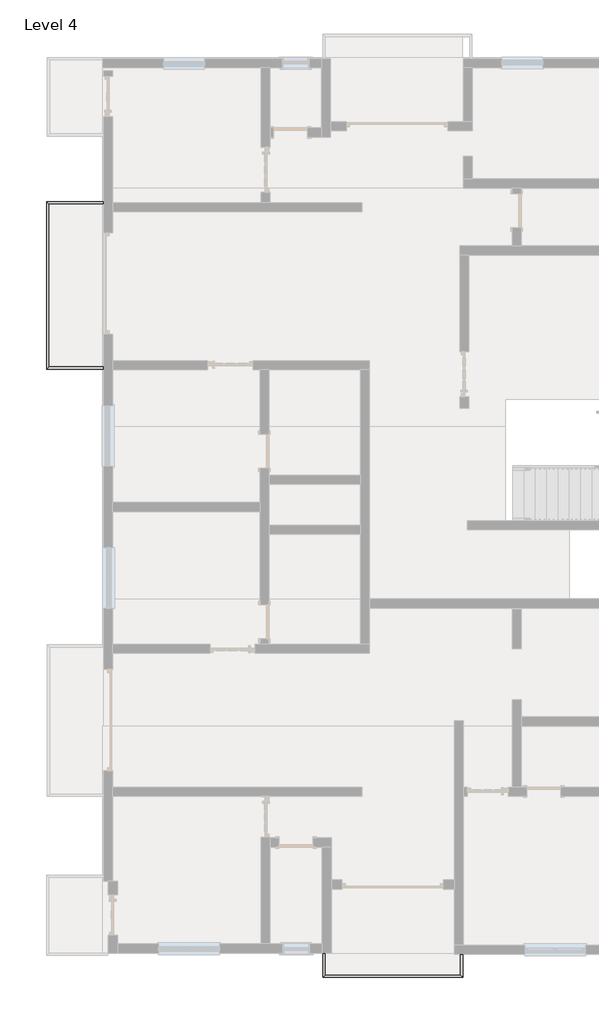
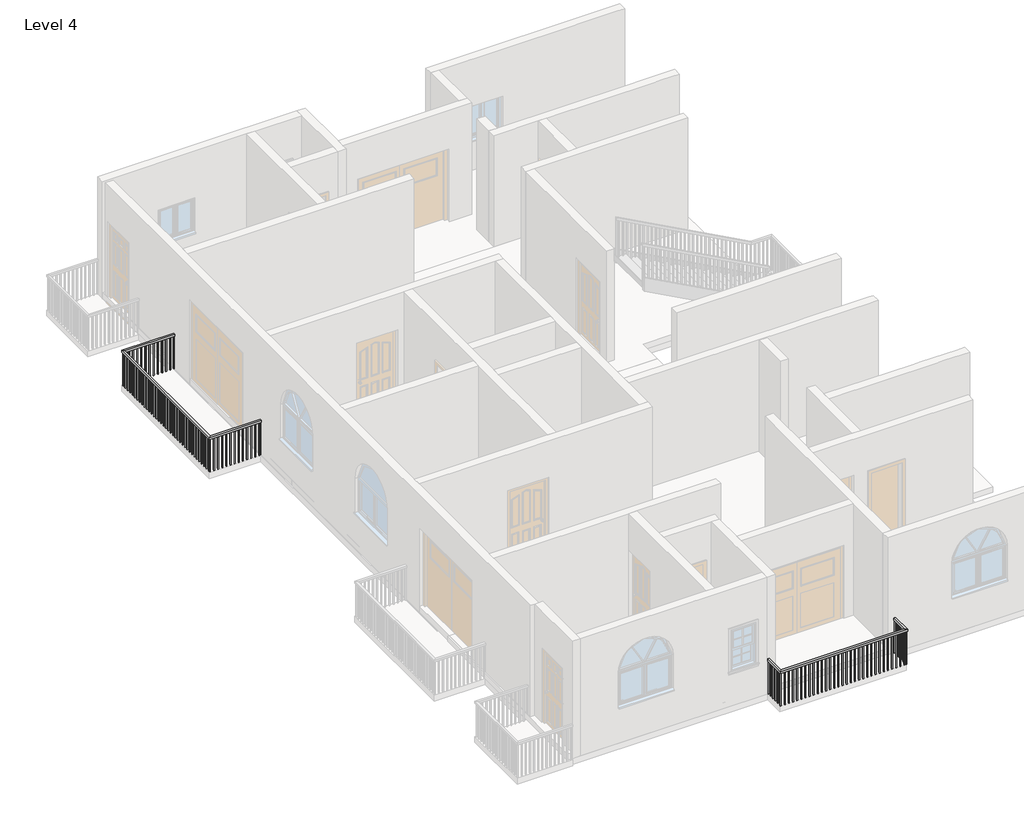
# One storey, part 4 of 7: 2 railings.
"""IFC4 building model written with IfcOpenShell, lengths in millimetres."""

from ifc_helpers import new_model, si_unit, frame, origin, place, context, project, spatial, polyline, outline, extrude, faceted_brep, element, save

model = new_model("IFC4")

# Units and contexts
model_context = context("Model", 3, world=origin())
ifc_project = project(units=[si_unit("LENGTHUNIT", "METRE", prefix="MILLI")], contexts=[model_context])

# Site, building, storey
site = spatial("IfcSite", under=ifc_project)
building = spatial("IfcBuilding", under=site)
storey = spatial("IfcBuildingStorey", under=building, Name="Level 4", Elevation=9144.0)

# Railings
placement = place(None, origin())
element("IfcRailing", 1, ObjectType="Handrail - Rectangular", at=placement, inside=storey, context=model_context, shape_type="SolidModel", body=[
    faceted_brep([(-1375.8109037, -10612.9037749, 10058.4), (-1375.8109037, -10612.9037749, 10007.6), (-1426.6109037, -10612.9037749, 10007.6), (-1426.6109037, -10612.9037749, 10058.4), (-1375.8109037, -11108.2037749, 10058.4), (-1375.8109037, -11108.2037749, 10007.6), (-1426.6109037, -11159.0037749, 10007.6), (-1426.6109037, -11159.0037749, 10058.4), (1659.4890963, -11108.2037749, 10058.4), (1659.4890963, -11108.2037749, 10007.6), (1710.2890963, -11159.0037749, 10007.6), (1710.2890963, -11159.0037749, 10058.4), (1659.4890963, -10638.3037749, 10058.4), (1710.2890963, -10638.3037749, 10058.4), (1710.2890963, -10638.3037749, 10007.6), (1659.4890963, -10638.3037749, 10007.6)], [[[0, 1, 2, 3]], [[1, 0, 4, 5]], [[2, 1, 5, 6]], [[3, 2, 6, 7]], [[0, 3, 7, 4]], [[5, 4, 8, 9]], [[6, 5, 9, 10]], [[7, 6, 10, 11]], [[4, 7, 11, 8]], [[12, 13, 14, 15]], [[9, 8, 12, 15]], [[10, 9, 15, 14]], [[11, 10, 14, 13]], [[8, 11, 13, 12]]]),
    extrude(outline(polyline([(1694.4140963, -10736.7287749), (1675.3640963, -10736.7287749), (1675.3640963, -10717.6787749), (1694.4140963, -10717.6787749), (1694.4140963, -10736.7287749)])), frame((0.0, 0.0, 9144.0), z_axis=(0.0, 0.0, 1.0), x_axis=(1.0, 0.0, 0.0)), (0.0, 0.0, 1.0), 863.6),
    extrude(outline(polyline([(1694.4140963, -10838.3287749), (1675.3640963, -10838.3287749), (1675.3640963, -10819.2787749), (1694.4140963, -10819.2787749), (1694.4140963, -10838.3287749)])), frame((0.0, 0.0, 9144.0), z_axis=(0.0, 0.0, 1.0), x_axis=(1.0, 0.0, 0.0)), (0.0, 0.0, 1.0), 863.6),
    extrude(outline(polyline([(1694.4140963, -10939.9287749), (1675.3640963, -10939.9287749), (1675.3640963, -10920.8787749), (1694.4140963, -10920.8787749), (1694.4140963, -10939.9287749)])), frame((0.0, 0.0, 9144.0), z_axis=(0.0, 0.0, 1.0), x_axis=(1.0, 0.0, 0.0)), (0.0, 0.0, 1.0), 863.6),
    extrude(outline(polyline([(1694.4140963, -11041.5287749), (1675.3640963, -11041.5287749), (1675.3640963, -11022.4787749), (1694.4140963, -11022.4787749), (1694.4140963, -11041.5287749)])), frame((0.0, 0.0, 9144.0), z_axis=(0.0, 0.0, 1.0), x_axis=(1.0, 0.0, 0.0)), (0.0, 0.0, 1.0), 863.6),
    extrude(outline(polyline([(1637.2640963, -11143.1287749), (1637.2640963, -11124.0787749), (1656.3140963, -11124.0787749), (1656.3140963, -11143.1287749), (1637.2640963, -11143.1287749)])), frame((0.0, 0.0, 9144.0), z_axis=(0.0, 0.0, 1.0), x_axis=(1.0, 0.0, 0.0)), (0.0, 0.0, 1.0), 863.6),
    extrude(outline(polyline([(1535.6640963, -11143.1287749), (1535.6640963, -11124.0787749), (1554.7140963, -11124.0787749), (1554.7140963, -11143.1287749), (1535.6640963, -11143.1287749)])), frame((0.0, 0.0, 9144.0), z_axis=(0.0, 0.0, 1.0), x_axis=(1.0, 0.0, 0.0)), (0.0, 0.0, 1.0), 863.6),
    extrude(outline(polyline([(1434.0640963, -11143.1287749), (1434.0640963, -11124.0787749), (1453.1140963, -11124.0787749), (1453.1140963, -11143.1287749), (1434.0640963, -11143.1287749)])), frame((0.0, 0.0, 9144.0), z_axis=(0.0, 0.0, 1.0), x_axis=(1.0, 0.0, 0.0)), (0.0, 0.0, 1.0), 863.6),
    extrude(outline(polyline([(1332.4640963, -11143.1287749), (1332.4640963, -11124.0787749), (1351.5140963, -11124.0787749), (1351.5140963, -11143.1287749), (1332.4640963, -11143.1287749)])), frame((0.0, 0.0, 9144.0), z_axis=(0.0, 0.0, 1.0), x_axis=(1.0, 0.0, 0.0)), (0.0, 0.0, 1.0), 863.6),
    extrude(outline(polyline([(1230.8640963, -11143.1287749), (1230.8640963, -11124.0787749), (1249.9140963, -11124.0787749), (1249.9140963, -11143.1287749), (1230.8640963, -11143.1287749)])), frame((0.0, 0.0, 9144.0), z_axis=(0.0, 0.0, 1.0), x_axis=(1.0, 0.0, 0.0)), (0.0, 0.0, 1.0), 863.6),
    extrude(outline(polyline([(1129.2640963, -11143.1287749), (1129.2640963, -11124.0787749), (1148.3140963, -11124.0787749), (1148.3140963, -11143.1287749), (1129.2640963, -11143.1287749)])), frame((0.0, 0.0, 9144.0), z_axis=(0.0, 0.0, 1.0), x_axis=(1.0, 0.0, 0.0)), (0.0, 0.0, 1.0), 863.6),
    extrude(outline(polyline([(1027.6640963, -11143.1287749), (1027.6640963, -11124.0787749), (1046.7140963, -11124.0787749), (1046.7140963, -11143.1287749), (1027.6640963, -11143.1287749)])), frame((0.0, 0.0, 9144.0), z_axis=(0.0, 0.0, 1.0), x_axis=(1.0, 0.0, 0.0)), (0.0, 0.0, 1.0), 863.6),
    extrude(outline(polyline([(926.0640963, -11143.1287749), (926.0640963, -11124.0787749), (945.1140963, -11124.0787749), (945.1140963, -11143.1287749), (926.0640963, -11143.1287749)])), frame((0.0, 0.0, 9144.0), z_axis=(0.0, 0.0, 1.0), x_axis=(1.0, 0.0, 0.0)), (0.0, 0.0, 1.0), 863.6),
    extrude(outline(polyline([(824.4640963, -11143.1287749), (824.4640963, -11124.0787749), (843.5140963, -11124.0787749), (843.5140963, -11143.1287749), (824.4640963, -11143.1287749)])), frame((0.0, 0.0, 9144.0), z_axis=(0.0, 0.0, 1.0), x_axis=(1.0, 0.0, 0.0)), (0.0, 0.0, 1.0), 863.6),
    extrude(outline(polyline([(722.8640963, -11143.1287749), (722.8640963, -11124.0787749), (741.9140963, -11124.0787749), (741.9140963, -11143.1287749), (722.8640963, -11143.1287749)])), frame((0.0, 0.0, 9144.0), z_axis=(0.0, 0.0, 1.0), x_axis=(1.0, 0.0, 0.0)), (0.0, 0.0, 1.0), 863.6),
    extrude(outline(polyline([(621.2640963, -11143.1287749), (621.2640963, -11124.0787749), (640.3140963, -11124.0787749), (640.3140963, -11143.1287749), (621.2640963, -11143.1287749)])), frame((0.0, 0.0, 9144.0), z_axis=(0.0, 0.0, 1.0), x_axis=(1.0, 0.0, 0.0)), (0.0, 0.0, 1.0), 863.6),
    extrude(outline(polyline([(519.6640963, -11143.1287749), (519.6640963, -11124.0787749), (538.7140963, -11124.0787749), (538.7140963, -11143.1287749), (519.6640963, -11143.1287749)])), frame((0.0, 0.0, 9144.0), z_axis=(0.0, 0.0, 1.0), x_axis=(1.0, 0.0, 0.0)), (0.0, 0.0, 1.0), 863.6),
    extrude(outline(polyline([(418.0640963, -11143.1287749), (418.0640963, -11124.0787749), (437.1140963, -11124.0787749), (437.1140963, -11143.1287749), (418.0640963, -11143.1287749)])), frame((0.0, 0.0, 9144.0), z_axis=(0.0, 0.0, 1.0), x_axis=(1.0, 0.0, 0.0)), (0.0, 0.0, 1.0), 863.6),
    extrude(outline(polyline([(316.4640963, -11143.1287749), (316.4640963, -11124.0787749), (335.5140963, -11124.0787749), (335.5140963, -11143.1287749), (316.4640963, -11143.1287749)])), frame((0.0, 0.0, 9144.0), z_axis=(0.0, 0.0, 1.0), x_axis=(1.0, 0.0, 0.0)), (0.0, 0.0, 1.0), 863.6),
    extrude(outline(polyline([(214.8640963, -11143.1287749), (214.8640963, -11124.0787749), (233.9140963, -11124.0787749), (233.9140963, -11143.1287749), (214.8640963, -11143.1287749)])), frame((0.0, 0.0, 9144.0), z_axis=(0.0, 0.0, 1.0), x_axis=(1.0, 0.0, 0.0)), (0.0, 0.0, 1.0), 863.6),
    extrude(outline(polyline([(113.2640963, -11143.1287749), (113.2640963, -11124.0787749), (132.3140963, -11124.0787749), (132.3140963, -11143.1287749), (113.2640963, -11143.1287749)])), frame((0.0, 0.0, 9144.0), z_axis=(0.0, 0.0, 1.0), x_axis=(1.0, 0.0, 0.0)), (0.0, 0.0, 1.0), 863.6),
    extrude(outline(polyline([(11.6640963, -11143.1287749), (11.6640963, -11124.0787749), (30.7140963, -11124.0787749), (30.7140963, -11143.1287749), (11.6640963, -11143.1287749)])), frame((0.0, 0.0, 9144.0), z_axis=(0.0, 0.0, 1.0), x_axis=(1.0, 0.0, 0.0)), (0.0, 0.0, 1.0), 863.6),
    extrude(outline(polyline([(-89.9359037, -11143.1287749), (-89.9359037, -11124.0787749), (-70.8859037, -11124.0787749), (-70.8859037, -11143.1287749), (-89.9359037, -11143.1287749)])), frame((0.0, 0.0, 9144.0), z_axis=(0.0, 0.0, 1.0), x_axis=(1.0, 0.0, 0.0)), (0.0, 0.0, 1.0), 863.6),
    extrude(outline(polyline([(-191.5359037, -11143.1287749), (-191.5359037, -11124.0787749), (-172.4859037, -11124.0787749), (-172.4859037, -11143.1287749), (-191.5359037, -11143.1287749)])), frame((0.0, 0.0, 9144.0), z_axis=(0.0, 0.0, 1.0), x_axis=(1.0, 0.0, 0.0)), (0.0, 0.0, 1.0), 863.6),
    extrude(outline(polyline([(-293.1359037, -11143.1287749), (-293.1359037, -11124.0787749), (-274.0859037, -11124.0787749), (-274.0859037, -11143.1287749), (-293.1359037, -11143.1287749)])), frame((0.0, 0.0, 9144.0), z_axis=(0.0, 0.0, 1.0), x_axis=(1.0, 0.0, 0.0)), (0.0, 0.0, 1.0), 863.6),
    extrude(outline(polyline([(-394.7359037, -11143.1287749), (-394.7359037, -11124.0787749), (-375.6859037, -11124.0787749), (-375.6859037, -11143.1287749), (-394.7359037, -11143.1287749)])), frame((0.0, 0.0, 9144.0), z_axis=(0.0, 0.0, 1.0), x_axis=(1.0, 0.0, 0.0)), (0.0, 0.0, 1.0), 863.6),
    extrude(outline(polyline([(-496.3359037, -11143.1287749), (-496.3359037, -11124.0787749), (-477.2859037, -11124.0787749), (-477.2859037, -11143.1287749), (-496.3359037, -11143.1287749)])), frame((0.0, 0.0, 9144.0), z_axis=(0.0, 0.0, 1.0), x_axis=(1.0, 0.0, 0.0)), (0.0, 0.0, 1.0), 863.6),
    extrude(outline(polyline([(-597.9359037, -11143.1287749), (-597.9359037, -11124.0787749), (-578.8859037, -11124.0787749), (-578.8859037, -11143.1287749), (-597.9359037, -11143.1287749)])), frame((0.0, 0.0, 9144.0), z_axis=(0.0, 0.0, 1.0), x_axis=(1.0, 0.0, 0.0)), (0.0, 0.0, 1.0), 863.6),
    extrude(outline(polyline([(-699.5359037, -11143.1287749), (-699.5359037, -11124.0787749), (-680.4859037, -11124.0787749), (-680.4859037, -11143.1287749), (-699.5359037, -11143.1287749)])), frame((0.0, 0.0, 9144.0), z_axis=(0.0, 0.0, 1.0), x_axis=(1.0, 0.0, 0.0)), (0.0, 0.0, 1.0), 863.6),
    extrude(outline(polyline([(-801.1359037, -11143.1287749), (-801.1359037, -11124.0787749), (-782.0859037, -11124.0787749), (-782.0859037, -11143.1287749), (-801.1359037, -11143.1287749)])), frame((0.0, 0.0, 9144.0), z_axis=(0.0, 0.0, 1.0), x_axis=(1.0, 0.0, 0.0)), (0.0, 0.0, 1.0), 863.6),
    extrude(outline(polyline([(-902.7359037, -11143.1287749), (-902.7359037, -11124.0787749), (-883.6859037, -11124.0787749), (-883.6859037, -11143.1287749), (-902.7359037, -11143.1287749)])), frame((0.0, 0.0, 9144.0), z_axis=(0.0, 0.0, 1.0), x_axis=(1.0, 0.0, 0.0)), (0.0, 0.0, 1.0), 863.6),
    extrude(outline(polyline([(-1004.3359037, -11143.1287749), (-1004.3359037, -11124.0787749), (-985.2859037, -11124.0787749), (-985.2859037, -11143.1287749), (-1004.3359037, -11143.1287749)])), frame((0.0, 0.0, 9144.0), z_axis=(0.0, 0.0, 1.0), x_axis=(1.0, 0.0, 0.0)), (0.0, 0.0, 1.0), 863.6),
    extrude(outline(polyline([(-1105.9359037, -11143.1287749), (-1105.9359037, -11124.0787749), (-1086.8859037, -11124.0787749), (-1086.8859037, -11143.1287749), (-1105.9359037, -11143.1287749)])), frame((0.0, 0.0, 9144.0), z_axis=(0.0, 0.0, 1.0), x_axis=(1.0, 0.0, 0.0)), (0.0, 0.0, 1.0), 863.6),
    extrude(outline(polyline([(-1207.5359037, -11143.1287749), (-1207.5359037, -11124.0787749), (-1188.4859037, -11124.0787749), (-1188.4859037, -11143.1287749), (-1207.5359037, -11143.1287749)])), frame((0.0, 0.0, 9144.0), z_axis=(0.0, 0.0, 1.0), x_axis=(1.0, 0.0, 0.0)), (0.0, 0.0, 1.0), 863.6),
    extrude(outline(polyline([(-1309.1359037, -11143.1287749), (-1309.1359037, -11124.0787749), (-1290.0859037, -11124.0787749), (-1290.0859037, -11143.1287749), (-1309.1359037, -11143.1287749)])), frame((0.0, 0.0, 9144.0), z_axis=(0.0, 0.0, 1.0), x_axis=(1.0, 0.0, 0.0)), (0.0, 0.0, 1.0), 863.6),
    extrude(outline(polyline([(-1410.7359037, -11111.3787749), (-1391.6859037, -11111.3787749), (-1391.6859037, -11130.4287749), (-1410.7359037, -11130.4287749), (-1410.7359037, -11111.3787749)])), frame((0.0, 0.0, 9144.0), z_axis=(0.0, 0.0, 1.0), x_axis=(1.0, 0.0, 0.0)), (0.0, 0.0, 1.0), 863.6),
    extrude(outline(polyline([(-1410.7359037, -11009.7787749), (-1391.6859037, -11009.7787749), (-1391.6859037, -11028.8287749), (-1410.7359037, -11028.8287749), (-1410.7359037, -11009.7787749)])), frame((0.0, 0.0, 9144.0), z_axis=(0.0, 0.0, 1.0), x_axis=(1.0, 0.0, 0.0)), (0.0, 0.0, 1.0), 863.6),
    extrude(outline(polyline([(-1410.7359037, -10908.1787749), (-1391.6859037, -10908.1787749), (-1391.6859037, -10927.2287749), (-1410.7359037, -10927.2287749), (-1410.7359037, -10908.1787749)])), frame((0.0, 0.0, 9144.0), z_axis=(0.0, 0.0, 1.0), x_axis=(1.0, 0.0, 0.0)), (0.0, 0.0, 1.0), 863.6),
    extrude(outline(polyline([(-1410.7359037, -10806.5787749), (-1391.6859037, -10806.5787749), (-1391.6859037, -10825.6287749), (-1410.7359037, -10825.6287749), (-1410.7359037, -10806.5787749)])), frame((0.0, 0.0, 9144.0), z_axis=(0.0, 0.0, 1.0), x_axis=(1.0, 0.0, 0.0)), (0.0, 0.0, 1.0), 863.6),
    extrude(outline(polyline([(-1410.7359037, -10704.9787749), (-1391.6859037, -10704.9787749), (-1391.6859037, -10724.0287749), (-1410.7359037, -10724.0287749), (-1410.7359037, -10704.9787749)])), frame((0.0, 0.0, 9144.0), z_axis=(0.0, 0.0, 1.0), x_axis=(1.0, 0.0, 0.0)), (0.0, 0.0, 1.0), 863.6),
    extrude(outline(polyline([(1675.3640963, -11143.1287749), (1675.3640963, -11124.0787749), (1694.4140963, -11124.0787749), (1694.4140963, -11143.1287749), (1675.3640963, -11143.1287749)])), frame((0.0, 0.0, 9144.0), z_axis=(0.0, 0.0, 1.0), x_axis=(1.0, 0.0, 0.0)), (0.0, 0.0, 1.0), 863.6),
    extrude(outline(polyline([(-1410.7359037, -11124.0787749), (-1391.6859037, -11124.0787749), (-1391.6859037, -11143.1287749), (-1410.7359037, -11143.1287749), (-1410.7359037, -11124.0787749)])), frame((0.0, 0.0, 9144.0), z_axis=(0.0, 0.0, 1.0), x_axis=(1.0, 0.0, 0.0)), (0.0, 0.0, 1.0), 863.6),
    extrude(outline(polyline([(1694.4140963, -10657.3537749), (1675.3640963, -10657.3537749), (1675.3640963, -10638.3037749), (1694.4140963, -10638.3037749), (1694.4140963, -10657.3537749)])), frame((0.0, 0.0, 9144.0), z_axis=(0.0, 0.0, 1.0), x_axis=(1.0, 0.0, 0.0)), (0.0, 0.0, 1.0), 863.6),
    extrude(outline(polyline([(-1410.7359037, -10612.9037749), (-1391.6859037, -10612.9037749), (-1391.6859037, -10631.9537749), (-1410.7359037, -10631.9537749), (-1410.7359037, -10612.9037749)])), frame((0.0, 0.0, 9144.0), z_axis=(0.0, 0.0, 1.0), x_axis=(1.0, 0.0, 0.0)), (0.0, 0.0, 1.0), 863.6),
])
element("IfcRailing", 2, ObjectType="Handrail - Rectangular", at=placement, inside=storey, context=model_context, shape_type="SolidModel", body=[
    faceted_brep([(-6330.8013636, 6151.0962251, 10058.4), (-6330.8013636, 6151.0962251, 10007.6), (-6330.8013636, 6201.8962251, 10007.6), (-6330.8013636, 6201.8962251, 10058.4), (-7563.8859037, 6151.0962251, 10058.4), (-7563.8859037, 6151.0962251, 10007.6), (-7614.6859037, 6201.8962251, 10007.6), (-7614.6859037, 6201.8962251, 10058.4), (-7563.8859037, 2506.1962251, 10058.4), (-7563.8859037, 2506.1962251, 10007.6), (-7614.6859037, 2455.3962251, 10007.6), (-7614.6859037, 2455.3962251, 10058.4), (-6330.8013636, 2506.1962251, 10058.4), (-6330.8013636, 2455.3962251, 10058.4), (-6330.8013636, 2455.3962251, 10007.6), (-6330.8013636, 2506.1962251, 10007.6)], [[[0, 1, 2, 3]], [[1, 0, 4, 5]], [[2, 1, 5, 6]], [[3, 2, 6, 7]], [[0, 3, 7, 4]], [[5, 4, 8, 9]], [[6, 5, 9, 10]], [[7, 6, 10, 11]], [[4, 7, 11, 8]], [[12, 13, 14, 15]], [[9, 8, 12, 15]], [[10, 9, 15, 14]], [[11, 10, 14, 13]], [[8, 11, 13, 12]]]),
    extrude(outline(polyline([(-6379.6109037, 2471.2712251), (-6379.6109037, 2490.3212251), (-6360.5609037, 2490.3212251), (-6360.5609037, 2471.2712251), (-6379.6109037, 2471.2712251)])), frame((0.0, 0.0, 9144.0), z_axis=(0.0, 0.0, 1.0), x_axis=(1.0, 0.0, 0.0)), (0.0, 0.0, 1.0), 863.6),
    extrude(outline(polyline([(-6481.2109037, 2471.2712251), (-6481.2109037, 2490.3212251), (-6462.1609037, 2490.3212251), (-6462.1609037, 2471.2712251), (-6481.2109037, 2471.2712251)])), frame((0.0, 0.0, 9144.0), z_axis=(0.0, 0.0, 1.0), x_axis=(1.0, 0.0, 0.0)), (0.0, 0.0, 1.0), 863.6),
    extrude(outline(polyline([(-6582.8109037, 2471.2712251), (-6582.8109037, 2490.3212251), (-6563.7609037, 2490.3212251), (-6563.7609037, 2471.2712251), (-6582.8109037, 2471.2712251)])), frame((0.0, 0.0, 9144.0), z_axis=(0.0, 0.0, 1.0), x_axis=(1.0, 0.0, 0.0)), (0.0, 0.0, 1.0), 863.6),
    extrude(outline(polyline([(-6684.4109037, 2471.2712251), (-6684.4109037, 2490.3212251), (-6665.3609037, 2490.3212251), (-6665.3609037, 2471.2712251), (-6684.4109037, 2471.2712251)])), frame((0.0, 0.0, 9144.0), z_axis=(0.0, 0.0, 1.0), x_axis=(1.0, 0.0, 0.0)), (0.0, 0.0, 1.0), 863.6),
    extrude(outline(polyline([(-6786.0109037, 2471.2712251), (-6786.0109037, 2490.3212251), (-6766.9609037, 2490.3212251), (-6766.9609037, 2471.2712251), (-6786.0109037, 2471.2712251)])), frame((0.0, 0.0, 9144.0), z_axis=(0.0, 0.0, 1.0), x_axis=(1.0, 0.0, 0.0)), (0.0, 0.0, 1.0), 863.6),
    extrude(outline(polyline([(-6887.6109037, 2471.2712251), (-6887.6109037, 2490.3212251), (-6868.5609037, 2490.3212251), (-6868.5609037, 2471.2712251), (-6887.6109037, 2471.2712251)])), frame((0.0, 0.0, 9144.0), z_axis=(0.0, 0.0, 1.0), x_axis=(1.0, 0.0, 0.0)), (0.0, 0.0, 1.0), 863.6),
    extrude(outline(polyline([(-6989.2109037, 2471.2712251), (-6989.2109037, 2490.3212251), (-6970.1609037, 2490.3212251), (-6970.1609037, 2471.2712251), (-6989.2109037, 2471.2712251)])), frame((0.0, 0.0, 9144.0), z_axis=(0.0, 0.0, 1.0), x_axis=(1.0, 0.0, 0.0)), (0.0, 0.0, 1.0), 863.6),
    extrude(outline(polyline([(-7090.8109037, 2471.2712251), (-7090.8109037, 2490.3212251), (-7071.7609037, 2490.3212251), (-7071.7609037, 2471.2712251), (-7090.8109037, 2471.2712251)])), frame((0.0, 0.0, 9144.0), z_axis=(0.0, 0.0, 1.0), x_axis=(1.0, 0.0, 0.0)), (0.0, 0.0, 1.0), 863.6),
    extrude(outline(polyline([(-7192.4109037, 2471.2712251), (-7192.4109037, 2490.3212251), (-7173.3609037, 2490.3212251), (-7173.3609037, 2471.2712251), (-7192.4109037, 2471.2712251)])), frame((0.0, 0.0, 9144.0), z_axis=(0.0, 0.0, 1.0), x_axis=(1.0, 0.0, 0.0)), (0.0, 0.0, 1.0), 863.6),
    extrude(outline(polyline([(-7294.0109037, 2471.2712251), (-7294.0109037, 2490.3212251), (-7274.9609037, 2490.3212251), (-7274.9609037, 2471.2712251), (-7294.0109037, 2471.2712251)])), frame((0.0, 0.0, 9144.0), z_axis=(0.0, 0.0, 1.0), x_axis=(1.0, 0.0, 0.0)), (0.0, 0.0, 1.0), 863.6),
    extrude(outline(polyline([(-7395.6109037, 2471.2712251), (-7395.6109037, 2490.3212251), (-7376.5609037, 2490.3212251), (-7376.5609037, 2471.2712251), (-7395.6109037, 2471.2712251)])), frame((0.0, 0.0, 9144.0), z_axis=(0.0, 0.0, 1.0), x_axis=(1.0, 0.0, 0.0)), (0.0, 0.0, 1.0), 863.6),
    extrude(outline(polyline([(-7497.2109037, 2471.2712251), (-7497.2109037, 2490.3212251), (-7478.1609037, 2490.3212251), (-7478.1609037, 2471.2712251), (-7497.2109037, 2471.2712251)])), frame((0.0, 0.0, 9144.0), z_axis=(0.0, 0.0, 1.0), x_axis=(1.0, 0.0, 0.0)), (0.0, 0.0, 1.0), 863.6),
    extrude(outline(polyline([(-7598.8109037, 2528.4212251), (-7579.7609037, 2528.4212251), (-7579.7609037, 2509.3712251), (-7598.8109037, 2509.3712251), (-7598.8109037, 2528.4212251)])), frame((0.0, 0.0, 9144.0), z_axis=(0.0, 0.0, 1.0), x_axis=(1.0, 0.0, 0.0)), (0.0, 0.0, 1.0), 863.6),
    extrude(outline(polyline([(-7598.8109037, 2630.0212251), (-7579.7609037, 2630.0212251), (-7579.7609037, 2610.9712251), (-7598.8109037, 2610.9712251), (-7598.8109037, 2630.0212251)])), frame((0.0, 0.0, 9144.0), z_axis=(0.0, 0.0, 1.0), x_axis=(1.0, 0.0, 0.0)), (0.0, 0.0, 1.0), 863.6),
    extrude(outline(polyline([(-7598.8109037, 2731.6212251), (-7579.7609037, 2731.6212251), (-7579.7609037, 2712.5712251), (-7598.8109037, 2712.5712251), (-7598.8109037, 2731.6212251)])), frame((0.0, 0.0, 9144.0), z_axis=(0.0, 0.0, 1.0), x_axis=(1.0, 0.0, 0.0)), (0.0, 0.0, 1.0), 863.6),
    extrude(outline(polyline([(-7598.8109037, 2833.2212251), (-7579.7609037, 2833.2212251), (-7579.7609037, 2814.1712251), (-7598.8109037, 2814.1712251), (-7598.8109037, 2833.2212251)])), frame((0.0, 0.0, 9144.0), z_axis=(0.0, 0.0, 1.0), x_axis=(1.0, 0.0, 0.0)), (0.0, 0.0, 1.0), 863.6),
    extrude(outline(polyline([(-7598.8109037, 2934.8212251), (-7579.7609037, 2934.8212251), (-7579.7609037, 2915.7712251), (-7598.8109037, 2915.7712251), (-7598.8109037, 2934.8212251)])), frame((0.0, 0.0, 9144.0), z_axis=(0.0, 0.0, 1.0), x_axis=(1.0, 0.0, 0.0)), (0.0, 0.0, 1.0), 863.6),
    extrude(outline(polyline([(-7598.8109037, 3036.4212251), (-7579.7609037, 3036.4212251), (-7579.7609037, 3017.3712251), (-7598.8109037, 3017.3712251), (-7598.8109037, 3036.4212251)])), frame((0.0, 0.0, 9144.0), z_axis=(0.0, 0.0, 1.0), x_axis=(1.0, 0.0, 0.0)), (0.0, 0.0, 1.0), 863.6),
    extrude(outline(polyline([(-7598.8109037, 3138.0212251), (-7579.7609037, 3138.0212251), (-7579.7609037, 3118.9712251), (-7598.8109037, 3118.9712251), (-7598.8109037, 3138.0212251)])), frame((0.0, 0.0, 9144.0), z_axis=(0.0, 0.0, 1.0), x_axis=(1.0, 0.0, 0.0)), (0.0, 0.0, 1.0), 863.6),
    extrude(outline(polyline([(-7598.8109037, 3239.6212251), (-7579.7609037, 3239.6212251), (-7579.7609037, 3220.5712251), (-7598.8109037, 3220.5712251), (-7598.8109037, 3239.6212251)])), frame((0.0, 0.0, 9144.0), z_axis=(0.0, 0.0, 1.0), x_axis=(1.0, 0.0, 0.0)), (0.0, 0.0, 1.0), 863.6),
    extrude(outline(polyline([(-7598.8109037, 3341.2212251), (-7579.7609037, 3341.2212251), (-7579.7609037, 3322.1712251), (-7598.8109037, 3322.1712251), (-7598.8109037, 3341.2212251)])), frame((0.0, 0.0, 9144.0), z_axis=(0.0, 0.0, 1.0), x_axis=(1.0, 0.0, 0.0)), (0.0, 0.0, 1.0), 863.6),
    extrude(outline(polyline([(-7598.8109037, 3442.8212251), (-7579.7609037, 3442.8212251), (-7579.7609037, 3423.7712251), (-7598.8109037, 3423.7712251), (-7598.8109037, 3442.8212251)])), frame((0.0, 0.0, 9144.0), z_axis=(0.0, 0.0, 1.0), x_axis=(1.0, 0.0, 0.0)), (0.0, 0.0, 1.0), 863.6),
    extrude(outline(polyline([(-7598.8109037, 3544.4212251), (-7579.7609037, 3544.4212251), (-7579.7609037, 3525.3712251), (-7598.8109037, 3525.3712251), (-7598.8109037, 3544.4212251)])), frame((0.0, 0.0, 9144.0), z_axis=(0.0, 0.0, 1.0), x_axis=(1.0, 0.0, 0.0)), (0.0, 0.0, 1.0), 863.6),
    extrude(outline(polyline([(-7598.8109037, 3646.0212251), (-7579.7609037, 3646.0212251), (-7579.7609037, 3626.9712251), (-7598.8109037, 3626.9712251), (-7598.8109037, 3646.0212251)])), frame((0.0, 0.0, 9144.0), z_axis=(0.0, 0.0, 1.0), x_axis=(1.0, 0.0, 0.0)), (0.0, 0.0, 1.0), 863.6),
    extrude(outline(polyline([(-7598.8109037, 3747.6212251), (-7579.7609037, 3747.6212251), (-7579.7609037, 3728.5712251), (-7598.8109037, 3728.5712251), (-7598.8109037, 3747.6212251)])), frame((0.0, 0.0, 9144.0), z_axis=(0.0, 0.0, 1.0), x_axis=(1.0, 0.0, 0.0)), (0.0, 0.0, 1.0), 863.6),
    extrude(outline(polyline([(-7598.8109037, 3849.2212251), (-7579.7609037, 3849.2212251), (-7579.7609037, 3830.1712251), (-7598.8109037, 3830.1712251), (-7598.8109037, 3849.2212251)])), frame((0.0, 0.0, 9144.0), z_axis=(0.0, 0.0, 1.0), x_axis=(1.0, 0.0, 0.0)), (0.0, 0.0, 1.0), 863.6),
    extrude(outline(polyline([(-7598.8109037, 3950.8212251), (-7579.7609037, 3950.8212251), (-7579.7609037, 3931.7712251), (-7598.8109037, 3931.7712251), (-7598.8109037, 3950.8212251)])), frame((0.0, 0.0, 9144.0), z_axis=(0.0, 0.0, 1.0), x_axis=(1.0, 0.0, 0.0)), (0.0, 0.0, 1.0), 863.6),
    extrude(outline(polyline([(-7598.8109037, 4052.4212251), (-7579.7609037, 4052.4212251), (-7579.7609037, 4033.3712251), (-7598.8109037, 4033.3712251), (-7598.8109037, 4052.4212251)])), frame((0.0, 0.0, 9144.0), z_axis=(0.0, 0.0, 1.0), x_axis=(1.0, 0.0, 0.0)), (0.0, 0.0, 1.0), 863.6),
    extrude(outline(polyline([(-7598.8109037, 4154.0212251), (-7579.7609037, 4154.0212251), (-7579.7609037, 4134.9712251), (-7598.8109037, 4134.9712251), (-7598.8109037, 4154.0212251)])), frame((0.0, 0.0, 9144.0), z_axis=(0.0, 0.0, 1.0), x_axis=(1.0, 0.0, 0.0)), (0.0, 0.0, 1.0), 863.6),
    extrude(outline(polyline([(-7598.8109037, 4255.6212251), (-7579.7609037, 4255.6212251), (-7579.7609037, 4236.5712251), (-7598.8109037, 4236.5712251), (-7598.8109037, 4255.6212251)])), frame((0.0, 0.0, 9144.0), z_axis=(0.0, 0.0, 1.0), x_axis=(1.0, 0.0, 0.0)), (0.0, 0.0, 1.0), 863.6),
    extrude(outline(polyline([(-7598.8109037, 4357.2212251), (-7579.7609037, 4357.2212251), (-7579.7609037, 4338.1712251), (-7598.8109037, 4338.1712251), (-7598.8109037, 4357.2212251)])), frame((0.0, 0.0, 9144.0), z_axis=(0.0, 0.0, 1.0), x_axis=(1.0, 0.0, 0.0)), (0.0, 0.0, 1.0), 863.6),
    extrude(outline(polyline([(-7598.8109037, 4458.8212251), (-7579.7609037, 4458.8212251), (-7579.7609037, 4439.7712251), (-7598.8109037, 4439.7712251), (-7598.8109037, 4458.8212251)])), frame((0.0, 0.0, 9144.0), z_axis=(0.0, 0.0, 1.0), x_axis=(1.0, 0.0, 0.0)), (0.0, 0.0, 1.0), 863.6),
    extrude(outline(polyline([(-7598.8109037, 4560.4212251), (-7579.7609037, 4560.4212251), (-7579.7609037, 4541.3712251), (-7598.8109037, 4541.3712251), (-7598.8109037, 4560.4212251)])), frame((0.0, 0.0, 9144.0), z_axis=(0.0, 0.0, 1.0), x_axis=(1.0, 0.0, 0.0)), (0.0, 0.0, 1.0), 863.6),
    extrude(outline(polyline([(-7598.8109037, 4662.0212251), (-7579.7609037, 4662.0212251), (-7579.7609037, 4642.9712251), (-7598.8109037, 4642.9712251), (-7598.8109037, 4662.0212251)])), frame((0.0, 0.0, 9144.0), z_axis=(0.0, 0.0, 1.0), x_axis=(1.0, 0.0, 0.0)), (0.0, 0.0, 1.0), 863.6),
    extrude(outline(polyline([(-7598.8109037, 4763.6212251), (-7579.7609037, 4763.6212251), (-7579.7609037, 4744.5712251), (-7598.8109037, 4744.5712251), (-7598.8109037, 4763.6212251)])), frame((0.0, 0.0, 9144.0), z_axis=(0.0, 0.0, 1.0), x_axis=(1.0, 0.0, 0.0)), (0.0, 0.0, 1.0), 863.6),
    extrude(outline(polyline([(-7598.8109037, 4865.2212251), (-7579.7609037, 4865.2212251), (-7579.7609037, 4846.1712251), (-7598.8109037, 4846.1712251), (-7598.8109037, 4865.2212251)])), frame((0.0, 0.0, 9144.0), z_axis=(0.0, 0.0, 1.0), x_axis=(1.0, 0.0, 0.0)), (0.0, 0.0, 1.0), 863.6),
    extrude(outline(polyline([(-7598.8109037, 4966.8212251), (-7579.7609037, 4966.8212251), (-7579.7609037, 4947.7712251), (-7598.8109037, 4947.7712251), (-7598.8109037, 4966.8212251)])), frame((0.0, 0.0, 9144.0), z_axis=(0.0, 0.0, 1.0), x_axis=(1.0, 0.0, 0.0)), (0.0, 0.0, 1.0), 863.6),
    extrude(outline(polyline([(-7598.8109037, 5068.4212251), (-7579.7609037, 5068.4212251), (-7579.7609037, 5049.3712251), (-7598.8109037, 5049.3712251), (-7598.8109037, 5068.4212251)])), frame((0.0, 0.0, 9144.0), z_axis=(0.0, 0.0, 1.0), x_axis=(1.0, 0.0, 0.0)), (0.0, 0.0, 1.0), 863.6),
    extrude(outline(polyline([(-7598.8109037, 5170.0212251), (-7579.7609037, 5170.0212251), (-7579.7609037, 5150.9712251), (-7598.8109037, 5150.9712251), (-7598.8109037, 5170.0212251)])), frame((0.0, 0.0, 9144.0), z_axis=(0.0, 0.0, 1.0), x_axis=(1.0, 0.0, 0.0)), (0.0, 0.0, 1.0), 863.6),
    extrude(outline(polyline([(-7598.8109037, 5271.6212251), (-7579.7609037, 5271.6212251), (-7579.7609037, 5252.5712251), (-7598.8109037, 5252.5712251), (-7598.8109037, 5271.6212251)])), frame((0.0, 0.0, 9144.0), z_axis=(0.0, 0.0, 1.0), x_axis=(1.0, 0.0, 0.0)), (0.0, 0.0, 1.0), 863.6),
    extrude(outline(polyline([(-7598.8109037, 5373.2212251), (-7579.7609037, 5373.2212251), (-7579.7609037, 5354.1712251), (-7598.8109037, 5354.1712251), (-7598.8109037, 5373.2212251)])), frame((0.0, 0.0, 9144.0), z_axis=(0.0, 0.0, 1.0), x_axis=(1.0, 0.0, 0.0)), (0.0, 0.0, 1.0), 863.6),
    extrude(outline(polyline([(-7598.8109037, 5474.8212251), (-7579.7609037, 5474.8212251), (-7579.7609037, 5455.7712251), (-7598.8109037, 5455.7712251), (-7598.8109037, 5474.8212251)])), frame((0.0, 0.0, 9144.0), z_axis=(0.0, 0.0, 1.0), x_axis=(1.0, 0.0, 0.0)), (0.0, 0.0, 1.0), 863.6),
    extrude(outline(polyline([(-7598.8109037, 5576.4212251), (-7579.7609037, 5576.4212251), (-7579.7609037, 5557.3712251), (-7598.8109037, 5557.3712251), (-7598.8109037, 5576.4212251)])), frame((0.0, 0.0, 9144.0), z_axis=(0.0, 0.0, 1.0), x_axis=(1.0, 0.0, 0.0)), (0.0, 0.0, 1.0), 863.6),
    extrude(outline(polyline([(-7598.8109037, 5678.0212251), (-7579.7609037, 5678.0212251), (-7579.7609037, 5658.9712251), (-7598.8109037, 5658.9712251), (-7598.8109037, 5678.0212251)])), frame((0.0, 0.0, 9144.0), z_axis=(0.0, 0.0, 1.0), x_axis=(1.0, 0.0, 0.0)), (0.0, 0.0, 1.0), 863.6),
    extrude(outline(polyline([(-7598.8109037, 5779.6212251), (-7579.7609037, 5779.6212251), (-7579.7609037, 5760.5712251), (-7598.8109037, 5760.5712251), (-7598.8109037, 5779.6212251)])), frame((0.0, 0.0, 9144.0), z_axis=(0.0, 0.0, 1.0), x_axis=(1.0, 0.0, 0.0)), (0.0, 0.0, 1.0), 863.6),
    extrude(outline(polyline([(-7598.8109037, 5881.2212251), (-7579.7609037, 5881.2212251), (-7579.7609037, 5862.1712251), (-7598.8109037, 5862.1712251), (-7598.8109037, 5881.2212251)])), frame((0.0, 0.0, 9144.0), z_axis=(0.0, 0.0, 1.0), x_axis=(1.0, 0.0, 0.0)), (0.0, 0.0, 1.0), 863.6),
    extrude(outline(polyline([(-7598.8109037, 5982.8212251), (-7579.7609037, 5982.8212251), (-7579.7609037, 5963.7712251), (-7598.8109037, 5963.7712251), (-7598.8109037, 5982.8212251)])), frame((0.0, 0.0, 9144.0), z_axis=(0.0, 0.0, 1.0), x_axis=(1.0, 0.0, 0.0)), (0.0, 0.0, 1.0), 863.6),
    extrude(outline(polyline([(-7598.8109037, 6084.4212251), (-7579.7609037, 6084.4212251), (-7579.7609037, 6065.3712251), (-7598.8109037, 6065.3712251), (-7598.8109037, 6084.4212251)])), frame((0.0, 0.0, 9144.0), z_axis=(0.0, 0.0, 1.0), x_axis=(1.0, 0.0, 0.0)), (0.0, 0.0, 1.0), 863.6),
    extrude(outline(polyline([(-7540.4763636, 6186.0212251), (-7540.4763636, 6166.9712251), (-7559.5263636, 6166.9712251), (-7559.5263636, 6186.0212251), (-7540.4763636, 6186.0212251)])), frame((0.0, 0.0, 9144.0), z_axis=(0.0, 0.0, 1.0), x_axis=(1.0, 0.0, 0.0)), (0.0, 0.0, 1.0), 863.6),
    extrude(outline(polyline([(-7438.8763636, 6186.0212251), (-7438.8763636, 6166.9712251), (-7457.9263636, 6166.9712251), (-7457.9263636, 6186.0212251), (-7438.8763636, 6186.0212251)])), frame((0.0, 0.0, 9144.0), z_axis=(0.0, 0.0, 1.0), x_axis=(1.0, 0.0, 0.0)), (0.0, 0.0, 1.0), 863.6),
    extrude(outline(polyline([(-7337.2763636, 6186.0212251), (-7337.2763636, 6166.9712251), (-7356.3263636, 6166.9712251), (-7356.3263636, 6186.0212251), (-7337.2763636, 6186.0212251)])), frame((0.0, 0.0, 9144.0), z_axis=(0.0, 0.0, 1.0), x_axis=(1.0, 0.0, 0.0)), (0.0, 0.0, 1.0), 863.6),
    extrude(outline(polyline([(-7235.6763636, 6186.0212251), (-7235.6763636, 6166.9712251), (-7254.7263636, 6166.9712251), (-7254.7263636, 6186.0212251), (-7235.6763636, 6186.0212251)])), frame((0.0, 0.0, 9144.0), z_axis=(0.0, 0.0, 1.0), x_axis=(1.0, 0.0, 0.0)), (0.0, 0.0, 1.0), 863.6),
    extrude(outline(polyline([(-7134.0763636, 6186.0212251), (-7134.0763636, 6166.9712251), (-7153.1263636, 6166.9712251), (-7153.1263636, 6186.0212251), (-7134.0763636, 6186.0212251)])), frame((0.0, 0.0, 9144.0), z_axis=(0.0, 0.0, 1.0), x_axis=(1.0, 0.0, 0.0)), (0.0, 0.0, 1.0), 863.6),
    extrude(outline(polyline([(-7032.4763636, 6186.0212251), (-7032.4763636, 6166.9712251), (-7051.5263636, 6166.9712251), (-7051.5263636, 6186.0212251), (-7032.4763636, 6186.0212251)])), frame((0.0, 0.0, 9144.0), z_axis=(0.0, 0.0, 1.0), x_axis=(1.0, 0.0, 0.0)), (0.0, 0.0, 1.0), 863.6),
    extrude(outline(polyline([(-6930.8763636, 6186.0212251), (-6930.8763636, 6166.9712251), (-6949.9263636, 6166.9712251), (-6949.9263636, 6186.0212251), (-6930.8763636, 6186.0212251)])), frame((0.0, 0.0, 9144.0), z_axis=(0.0, 0.0, 1.0), x_axis=(1.0, 0.0, 0.0)), (0.0, 0.0, 1.0), 863.6),
    extrude(outline(polyline([(-6829.2763636, 6186.0212251), (-6829.2763636, 6166.9712251), (-6848.3263636, 6166.9712251), (-6848.3263636, 6186.0212251), (-6829.2763636, 6186.0212251)])), frame((0.0, 0.0, 9144.0), z_axis=(0.0, 0.0, 1.0), x_axis=(1.0, 0.0, 0.0)), (0.0, 0.0, 1.0), 863.6),
    extrude(outline(polyline([(-6727.6763636, 6186.0212251), (-6727.6763636, 6166.9712251), (-6746.7263636, 6166.9712251), (-6746.7263636, 6186.0212251), (-6727.6763636, 6186.0212251)])), frame((0.0, 0.0, 9144.0), z_axis=(0.0, 0.0, 1.0), x_axis=(1.0, 0.0, 0.0)), (0.0, 0.0, 1.0), 863.6),
    extrude(outline(polyline([(-6626.0763636, 6186.0212251), (-6626.0763636, 6166.9712251), (-6645.1263636, 6166.9712251), (-6645.1263636, 6186.0212251), (-6626.0763636, 6186.0212251)])), frame((0.0, 0.0, 9144.0), z_axis=(0.0, 0.0, 1.0), x_axis=(1.0, 0.0, 0.0)), (0.0, 0.0, 1.0), 863.6),
    extrude(outline(polyline([(-6524.4763636, 6186.0212251), (-6524.4763636, 6166.9712251), (-6543.5263636, 6166.9712251), (-6543.5263636, 6186.0212251), (-6524.4763636, 6186.0212251)])), frame((0.0, 0.0, 9144.0), z_axis=(0.0, 0.0, 1.0), x_axis=(1.0, 0.0, 0.0)), (0.0, 0.0, 1.0), 863.6),
    extrude(outline(polyline([(-6422.8763636, 6186.0212251), (-6422.8763636, 6166.9712251), (-6441.9263636, 6166.9712251), (-6441.9263636, 6186.0212251), (-6422.8763636, 6186.0212251)])), frame((0.0, 0.0, 9144.0), z_axis=(0.0, 0.0, 1.0), x_axis=(1.0, 0.0, 0.0)), (0.0, 0.0, 1.0), 863.6),
    extrude(outline(polyline([(-7598.8109037, 2490.3212251), (-7579.7609037, 2490.3212251), (-7579.7609037, 2471.2712251), (-7598.8109037, 2471.2712251), (-7598.8109037, 2490.3212251)])), frame((0.0, 0.0, 9144.0), z_axis=(0.0, 0.0, 1.0), x_axis=(1.0, 0.0, 0.0)), (0.0, 0.0, 1.0), 863.6),
    extrude(outline(polyline([(-7579.7609037, 6186.0212251), (-7579.7609037, 6166.9712251), (-7598.8109037, 6166.9712251), (-7598.8109037, 6186.0212251), (-7579.7609037, 6186.0212251)])), frame((0.0, 0.0, 9144.0), z_axis=(0.0, 0.0, 1.0), x_axis=(1.0, 0.0, 0.0)), (0.0, 0.0, 1.0), 863.6),
    extrude(outline(polyline([(-6349.8513636, 2471.2712251), (-6349.8513636, 2490.3212251), (-6330.8013636, 2490.3212251), (-6330.8013636, 2471.2712251), (-6349.8513636, 2471.2712251)])), frame((0.0, 0.0, 9144.0), z_axis=(0.0, 0.0, 1.0), x_axis=(1.0, 0.0, 0.0)), (0.0, 0.0, 1.0), 863.6),
    extrude(outline(polyline([(-6330.8013636, 6186.0212251), (-6330.8013636, 6166.9712251), (-6349.8513636, 6166.9712251), (-6349.8513636, 6186.0212251), (-6330.8013636, 6186.0212251)])), frame((0.0, 0.0, 9144.0), z_axis=(0.0, 0.0, 1.0), x_axis=(1.0, 0.0, 0.0)), (0.0, 0.0, 1.0), 863.6),
])

save(model, "model.ifc")

# Revit data of these elements
# Type "Handrail - Rectangular"
#   Assembly Code = "C2010400"
#   built-in parameter 1008612 = 0.0416667 (stored number, unit not read)
#   built-in parameter 1008611 = 0.0416667 (stored number, unit not read)
#   built-in parameter 1008609 = 0.333333 (stored number, unit not read)
#   built-in parameter 1008604 = 0.166667 (stored number, unit not read)
#   built-in parameter 1008603 = 0.166667 (stored number, unit not read)
#   Railing Height = 3' - 0"
#   built-in parameter 1008630 = 2
#   built-in parameter 1008610 = 2
#   built-in parameter 1008618 = Baluster - Square : 3/4"
# Elements 1, 2 (IfcRailing, "Handrail - Rectangular")
#   Phase Created = New Construction
